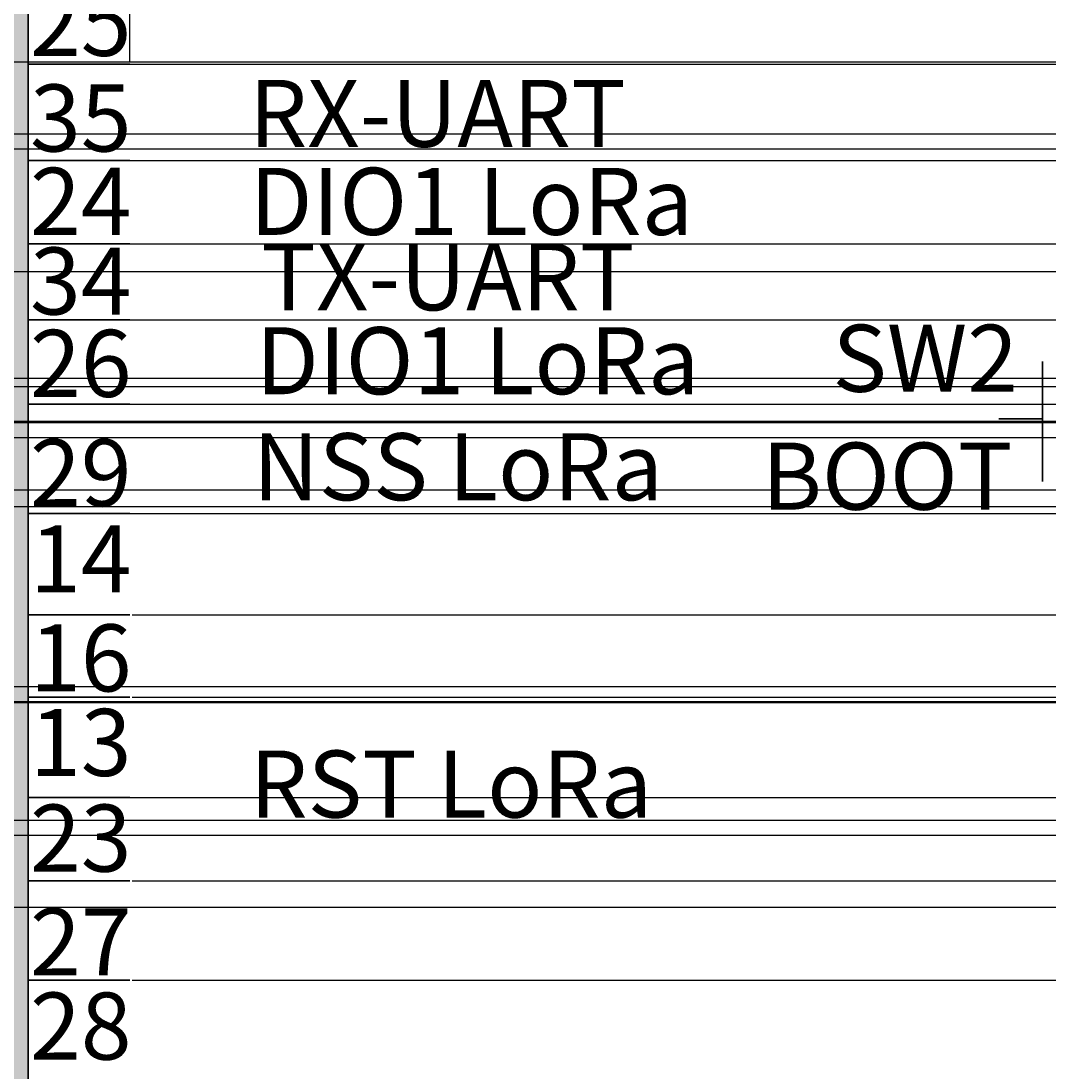
# Model space of a CAD drawing. Units: inches. Extents: x 23 to 132, y 5 to 105.
# Tile 10 of 14: x 81 to 107, y 50 to 77. Entities that reach past the tile are written whole.
import ezdxf

# ---------------------------------------------------------------- set-up
doc = ezdxf.new("R2010")
doc.units = ezdxf.units.IN
doc.header["$MEASUREMENT"] = 0
for name, color, linetype, lineweight in [('A-ANNO-DIMS', 2, 'Continuous', 18), ('E-ANNO-IDEN', 4, 'Continuous', 18), ('E-ANNO-NETL', 30, 'Continuous', 18), ('E-ANNO-TEXT', 3, 'Continuous', 18), ('E-SYMB', 1, 'Continuous', 35), ('E-SYMB-PATT', 1, 'Continuous', 18), ('E-WIRE', 3, 'Continuous', 25)]:
    doc.layers.add(name, color=color, linetype=linetype, lineweight=lineweight)
doc.styles.get("Standard").update_dxf_attribs({"font": 'arial.ttf'})
doc.dimstyles.get("Standard").update_dxf_attribs({"dimtxt": 0.18, "dimasz": 0.18, "dimexe": 0.18, "dimexo": 0.0625, "dimgap": 0.09, "dimtad": 0, "dimtih": 1, "dimtoh": 1, "dimdec": 4, "dimzin": 0, "dimdsep": 46, "dimtxsty": 'Standard', "dimcen": 0.09, "dimadec": 0, "dimazin": 0, "dimtfac": 1, "dimtdec": 4, "dimtofl": 0, "dimtmove": 0, "dimatfit": 3, "dimfxl": 1, "dimtolj": 1, "dimtzin": 0, "dimarcsym": 0})

# ---------------------------------------------------------------- blocks, each defined once
blk = doc.blocks.new('*D2')
at = {"layer": 'A-ANNO-DIMS', "color": 0, "lineweight": -2, "transparency": 16777216}
for p, q in [((28.697, 66.272), (28.697, 105.232)), ((123.211, 99.539), (123.211, 105.232)), ((28.877, 105.052), (75.577, 105.052)), ((123.031, 105.052), (76.33, 105.052))]:
    blk.add_line(p, q, dxfattribs=at)
at = {"layer": 'A-ANNO-DIMS', "color": 0, "transparency": 16777216}
for points in [[(28.877, 105.082), (28.877, 105.022), (28.697, 105.052)], [(123.031, 105.082), (123.031, 105.022), (123.211, 105.052)]]:
    blk.add_solid(points, dxfattribs=at)
at = {"layer": 'Defpoints', "color": 0, "transparency": 16777216}
for p in [(123.211, 105.052), (123.211, 99.477), (28.697, 66.21)]:
    blk.add_point(p, dxfattribs=at)
at = {"layer": 'A-ANNO-DIMS', "color": 0, "transparency": 16777216, "insert": (75.954, 105.052), "char_height": 0.18, "attachment_point": 5}
blk.add_mtext('\\A1;94.51', dxfattribs=at)
blk = doc.blocks.new('*D3')
at = {"layer": 'A-ANNO-DIMS', "color": 0, "lineweight": -2, "transparency": 16777216}
for p, q in [((121.409, 99.285), (129.239, 99.285)), ((129.059, 99.105), (129.059, 55.423)), ((129.059, 11.378), (129.059, 55.06)), ((72.981, 11.198), (129.239, 11.198))]:
    blk.add_line(p, q, dxfattribs=at)
at = {"layer": 'A-ANNO-DIMS', "color": 0, "transparency": 16777216}
for points in [[(129.029, 99.105), (129.089, 99.105), (129.059, 99.285)], [(129.029, 11.378), (129.089, 11.378), (129.059, 11.198)]]:
    blk.add_solid(points, dxfattribs=at)
at = {"layer": 'Defpoints', "color": 0, "transparency": 16777216}
for p in [(121.346, 99.285), (129.059, 99.285), (72.919, 11.198)]:
    blk.add_point(p, dxfattribs=at)
at = {"layer": 'A-ANNO-DIMS', "color": 0, "transparency": 16777216, "insert": (129.059, 55.241), "char_height": 0.18, "attachment_point": 5}
blk.add_mtext('\\A1;88.09', dxfattribs=at)
blk = doc.blocks.new('*D15')
at = {"layer": 'A-ANNO-DIMS', "color": 0, "lineweight": -2, "transparency": 16777216}
for p, q in [((50.327, 77.095), (129.239, 77.095)), ((129.059, 76.915), (129.059, 76.538)), ((129.059, 75.801), (129.059, 76.177)), ((47.783, 75.621), (129.239, 75.621))]:
    blk.add_line(p, q, dxfattribs=at)
at = {"layer": 'A-ANNO-DIMS', "color": 0, "transparency": 16777216}
for points in [[(129.029, 76.915), (129.089, 76.915), (129.059, 77.095)], [(129.029, 75.801), (129.089, 75.801), (129.059, 75.621)]]:
    blk.add_solid(points, dxfattribs=at)
at = {"layer": 'Defpoints', "color": 0, "transparency": 16777216}
for p in [(50.265, 77.095), (47.72, 75.621), (129.059, 75.621)]:
    blk.add_point(p, dxfattribs=at)
at = {"layer": 'A-ANNO-DIMS', "color": 0, "transparency": 16777216, "insert": (129.059, 76.358), "char_height": 0.18, "attachment_point": 5}
blk.add_mtext('\\A1;1.47', dxfattribs=at)
blk = doc.blocks.new('*D16')
at = {"layer": 'A-ANNO-DIMS', "color": 0, "lineweight": -2, "transparency": 16777216}
for p, q in [((47.783, 75.621), (129.239, 75.621)), ((129.059, 75.441), (129.059, 73.177)), ((129.059, 70.55), (129.059, 72.814)), ((47.783, 70.37), (129.239, 70.37))]:
    blk.add_line(p, q, dxfattribs=at)
at = {"layer": 'A-ANNO-DIMS', "color": 0, "transparency": 16777216}
for points in [[(129.029, 75.441), (129.089, 75.441), (129.059, 75.621)], [(129.029, 70.55), (129.089, 70.55), (129.059, 70.37)]]:
    blk.add_solid(points, dxfattribs=at)
at = {"layer": 'Defpoints', "color": 0, "transparency": 16777216}
for p in [(47.72, 75.621), (47.72, 70.37), (129.059, 70.37)]:
    blk.add_point(p, dxfattribs=at)
at = {"layer": 'A-ANNO-DIMS', "color": 0, "transparency": 16777216, "insert": (129.059, 72.996), "char_height": 0.18, "attachment_point": 5}
blk.add_mtext('\\A1;5.25', dxfattribs=at)
blk = doc.blocks.new('*D17')
at = {"layer": 'A-ANNO-DIMS', "color": 0, "lineweight": -2, "transparency": 16777216}
for p, q in [((47.783, 70.37), (129.239, 70.37)), ((129.059, 70.19), (129.059, 68.678)), ((129.059, 66.801), (129.059, 68.314)), ((47.783, 66.621), (129.239, 66.621))]:
    blk.add_line(p, q, dxfattribs=at)
at = {"layer": 'A-ANNO-DIMS', "color": 0, "transparency": 16777216}
for points in [[(129.029, 70.19), (129.089, 70.19), (129.059, 70.37)], [(129.029, 66.801), (129.089, 66.801), (129.059, 66.621)]]:
    blk.add_solid(points, dxfattribs=at)
at = {"layer": 'Defpoints', "color": 0, "transparency": 16777216}
for p in [(47.72, 70.37), (47.72, 66.621), (129.059, 66.621)]:
    blk.add_point(p, dxfattribs=at)
at = {"layer": 'A-ANNO-DIMS', "color": 0, "transparency": 16777216, "insert": (129.059, 68.496), "char_height": 0.18, "attachment_point": 5}
blk.add_mtext('\\A1;3.75', dxfattribs=at)
blk = doc.blocks.new('*D24')
at = {"layer": 'A-ANNO-DIMS', "color": 0, "lineweight": -2, "transparency": 16777216}
for p, q in [((81.032, 77.095), (129.239, 77.095)), ((129.059, 76.915), (129.059, 76.509)), ((129.059, 75.739), (129.059, 76.145)), ((83.576, 75.559), (129.239, 75.559))]:
    blk.add_line(p, q, dxfattribs=at)
at = {"layer": 'A-ANNO-DIMS', "color": 0, "transparency": 16777216}
for points in [[(129.029, 76.915), (129.089, 76.915), (129.059, 77.095)], [(129.029, 75.739), (129.089, 75.739), (129.059, 75.559)]]:
    blk.add_solid(points, dxfattribs=at)
at = {"layer": 'Defpoints', "color": 0, "transparency": 16777216}
for p in [(80.969, 77.095), (83.514, 75.559), (129.059, 75.559)]:
    blk.add_point(p, dxfattribs=at)
at = {"layer": 'A-ANNO-DIMS', "color": 0, "transparency": 16777216, "insert": (129.059, 76.327), "char_height": 0.18, "attachment_point": 5}
blk.add_mtext('\\A1;1.54', dxfattribs=at)
blk = doc.blocks.new('*D25')
at = {"layer": 'A-ANNO-DIMS', "color": 0, "lineweight": -2, "transparency": 16777216}
for p, q in [((83.576, 75.559), (129.239, 75.559)), ((129.059, 75.379), (129.059, 74.534)), ((129.059, 73.327), (129.059, 74.173)), ((83.576, 73.147), (129.239, 73.147))]:
    blk.add_line(p, q, dxfattribs=at)
at = {"layer": 'A-ANNO-DIMS', "color": 0, "transparency": 16777216}
for points in [[(129.029, 75.379), (129.089, 75.379), (129.059, 75.559)], [(129.029, 73.327), (129.089, 73.327), (129.059, 73.147)]]:
    blk.add_solid(points, dxfattribs=at)
at = {"layer": 'Defpoints', "color": 0, "transparency": 16777216}
for p in [(83.514, 75.559), (83.514, 73.147), (129.059, 73.147)]:
    blk.add_point(p, dxfattribs=at)
at = {"layer": 'A-ANNO-DIMS', "color": 0, "transparency": 16777216, "insert": (129.059, 74.353), "char_height": 0.18, "attachment_point": 5}
blk.add_mtext('\\A1;2.41', dxfattribs=at)
blk = doc.blocks.new('*D26')
at = {"layer": 'A-ANNO-DIMS', "color": 0, "lineweight": -2, "transparency": 16777216}
for p, q in [((83.576, 73.147), (129.239, 73.147)), ((129.059, 72.967), (129.059, 72.286)), ((129.059, 71.241), (129.059, 71.922)), ((83.576, 71.061), (129.239, 71.061))]:
    blk.add_line(p, q, dxfattribs=at)
at = {"layer": 'A-ANNO-DIMS', "color": 0, "transparency": 16777216}
for points in [[(129.029, 72.967), (129.089, 72.967), (129.059, 73.147)], [(129.029, 71.241), (129.089, 71.241), (129.059, 71.061)]]:
    blk.add_solid(points, dxfattribs=at)
at = {"layer": 'Defpoints', "color": 0, "transparency": 16777216}
for p in [(83.514, 73.147), (83.514, 71.061), (129.059, 71.061)]:
    blk.add_point(p, dxfattribs=at)
at = {"layer": 'A-ANNO-DIMS', "color": 0, "transparency": 16777216, "insert": (129.059, 72.104), "char_height": 0.18, "attachment_point": 5}
blk.add_mtext('\\A1;2.09', dxfattribs=at)
blk = doc.blocks.new('*D27')
at = {"layer": 'A-ANNO-DIMS', "color": 0, "lineweight": -2, "transparency": 16777216}
for p, q in [((83.576, 71.061), (129.239, 71.061)), ((129.059, 70.881), (129.059, 70.292)), ((129.059, 69.338), (129.059, 69.928)), ((83.576, 69.158), (129.239, 69.158))]:
    blk.add_line(p, q, dxfattribs=at)
at = {"layer": 'A-ANNO-DIMS', "color": 0, "transparency": 16777216}
for points in [[(129.029, 70.881), (129.089, 70.881), (129.059, 71.061)], [(129.029, 69.338), (129.089, 69.338), (129.059, 69.158)]]:
    blk.add_solid(points, dxfattribs=at)
at = {"layer": 'Defpoints', "color": 0, "transparency": 16777216}
for p in [(83.514, 71.061), (83.514, 69.158), (129.059, 69.158)]:
    blk.add_point(p, dxfattribs=at)
at = {"layer": 'A-ANNO-DIMS', "color": 0, "transparency": 16777216, "insert": (129.059, 70.11), "char_height": 0.18, "attachment_point": 5}
blk.add_mtext('\\A1;1.90', dxfattribs=at)
blk = doc.blocks.new('*D28')
at = {"layer": 'A-ANNO-DIMS', "color": 0, "lineweight": -2, "transparency": 16777216}
for p, q in [((83.576, 69.158), (129.239, 69.158)), ((129.059, 68.978), (129.059, 68.282)), ((129.059, 67.226), (129.059, 67.922)), ((83.576, 67.046), (129.239, 67.046))]:
    blk.add_line(p, q, dxfattribs=at)
at = {"layer": 'A-ANNO-DIMS', "color": 0, "transparency": 16777216}
for points in [[(129.029, 68.978), (129.089, 68.978), (129.059, 69.158)], [(129.029, 67.226), (129.089, 67.226), (129.059, 67.046)]]:
    blk.add_solid(points, dxfattribs=at)
at = {"layer": 'Defpoints', "color": 0, "transparency": 16777216}
for p in [(83.514, 69.158), (83.514, 67.046), (129.059, 67.046)]:
    blk.add_point(p, dxfattribs=at)
at = {"layer": 'A-ANNO-DIMS', "color": 0, "transparency": 16777216, "insert": (129.059, 68.102), "char_height": 0.18, "attachment_point": 5}
blk.add_mtext('\\A1;2.112', dxfattribs=at)
blk = doc.blocks.new('*D29')
at = {"layer": 'A-ANNO-DIMS', "color": 0, "lineweight": -2, "transparency": 16777216}
for p, q in [((83.576, 67.046), (129.239, 67.046)), ((129.059, 66.866), (129.059, 65.855)), ((129.059, 64.482), (129.059, 65.494)), ((83.576, 64.302), (129.239, 64.302))]:
    blk.add_line(p, q, dxfattribs=at)
at = {"layer": 'A-ANNO-DIMS', "color": 0, "transparency": 16777216}
for points in [[(129.029, 66.866), (129.089, 66.866), (129.059, 67.046)], [(129.029, 64.482), (129.089, 64.482), (129.059, 64.302)]]:
    blk.add_solid(points, dxfattribs=at)
at = {"layer": 'Defpoints', "color": 0, "transparency": 16777216}
for p in [(83.514, 67.046), (83.514, 64.302), (129.059, 64.302)]:
    blk.add_point(p, dxfattribs=at)
at = {"layer": 'A-ANNO-DIMS', "color": 0, "transparency": 16777216, "insert": (129.059, 65.674), "char_height": 0.18, "attachment_point": 5}
blk.add_mtext('\\A1;2.744', dxfattribs=at)
blk = doc.blocks.new('*D30')
at = {"layer": 'A-ANNO-DIMS', "color": 0, "lineweight": -2, "transparency": 16777216}
for p, q in [((83.576, 64.302), (129.239, 64.302)), ((129.059, 64.122), (129.059, 63.217)), ((129.059, 61.949), (129.059, 62.853)), ((83.576, 61.769), (129.239, 61.769))]:
    blk.add_line(p, q, dxfattribs=at)
at = {"layer": 'A-ANNO-DIMS', "color": 0, "transparency": 16777216}
for points in [[(129.029, 64.122), (129.089, 64.122), (129.059, 64.302)], [(129.029, 61.949), (129.089, 61.949), (129.059, 61.769)]]:
    blk.add_solid(points, dxfattribs=at)
at = {"layer": 'Defpoints', "color": 0, "transparency": 16777216}
for p in [(83.514, 64.302), (83.514, 61.769), (129.059, 61.769)]:
    blk.add_point(p, dxfattribs=at)
at = {"layer": 'A-ANNO-DIMS', "color": 0, "transparency": 16777216, "insert": (129.059, 63.035), "char_height": 0.18, "attachment_point": 5}
blk.add_mtext('\\A1;2.53', dxfattribs=at)
blk = doc.blocks.new('*D31')
at = {"layer": 'A-ANNO-DIMS', "color": 0, "lineweight": -2, "transparency": 16777216}
for p, q in [((83.576, 61.769), (129.239, 61.769)), ((129.059, 61.589), (129.059, 60.918)), ((129.059, 59.883), (129.059, 60.554)), ((83.576, 59.703), (129.239, 59.703))]:
    blk.add_line(p, q, dxfattribs=at)
at = {"layer": 'A-ANNO-DIMS', "color": 0, "transparency": 16777216}
for points in [[(129.029, 61.589), (129.089, 61.589), (129.059, 61.769)], [(129.029, 59.883), (129.089, 59.883), (129.059, 59.703)]]:
    blk.add_solid(points, dxfattribs=at)
at = {"layer": 'Defpoints', "color": 0, "transparency": 16777216}
for p in [(83.514, 61.769), (83.514, 59.703), (129.059, 59.703)]:
    blk.add_point(p, dxfattribs=at)
at = {"layer": 'A-ANNO-DIMS', "color": 0, "transparency": 16777216, "insert": (129.059, 60.736), "char_height": 0.18, "attachment_point": 5}
blk.add_mtext('\\A1;2.07', dxfattribs=at)
blk = doc.blocks.new('*D32')
at = {"layer": 'A-ANNO-DIMS', "color": 0, "lineweight": -2, "transparency": 16777216}
for p, q in [((83.576, 59.703), (129.239, 59.703)), ((129.059, 59.523), (129.059, 58.629)), ((129.059, 57.372), (129.059, 58.266)), ((83.576, 57.192), (129.239, 57.192))]:
    blk.add_line(p, q, dxfattribs=at)
at = {"layer": 'A-ANNO-DIMS', "color": 0, "transparency": 16777216}
for points in [[(129.029, 59.523), (129.089, 59.523), (129.059, 59.703)], [(129.029, 57.372), (129.089, 57.372), (129.059, 57.192)]]:
    blk.add_solid(points, dxfattribs=at)
at = {"layer": 'Defpoints', "color": 0, "transparency": 16777216}
for p in [(83.514, 59.703), (83.514, 57.192), (129.059, 57.192)]:
    blk.add_point(p, dxfattribs=at)
at = {"layer": 'A-ANNO-DIMS', "color": 0, "transparency": 16777216, "insert": (129.059, 58.447), "char_height": 0.18, "attachment_point": 5}
blk.add_mtext('\\A1;2.51', dxfattribs=at)
blk = doc.blocks.new('*D33')
at = {"layer": 'A-ANNO-DIMS', "color": 0, "lineweight": -2, "transparency": 16777216}
for p, q in [((83.576, 57.192), (129.239, 57.192)), ((129.059, 57.012), (129.059, 56.33)), ((129.059, 55.284), (129.059, 55.966)), ((83.576, 55.104), (129.239, 55.104))]:
    blk.add_line(p, q, dxfattribs=at)
at = {"layer": 'A-ANNO-DIMS', "color": 0, "transparency": 16777216}
for points in [[(129.029, 57.012), (129.089, 57.012), (129.059, 57.192)], [(129.029, 55.284), (129.089, 55.284), (129.059, 55.104)]]:
    blk.add_solid(points, dxfattribs=at)
at = {"layer": 'Defpoints', "color": 0, "transparency": 16777216}
for p in [(83.514, 57.192), (83.514, 55.104), (129.059, 55.104)]:
    blk.add_point(p, dxfattribs=at)
at = {"layer": 'A-ANNO-DIMS', "color": 0, "transparency": 16777216, "insert": (129.059, 56.148), "char_height": 0.18, "attachment_point": 5}
blk.add_mtext('\\A1;2.09', dxfattribs=at)
blk = doc.blocks.new('*D34')
at = {"layer": 'A-ANNO-DIMS', "color": 0, "lineweight": -2, "transparency": 16777216}
for p, q in [((83.576, 55.104), (129.239, 55.104)), ((129.059, 54.924), (129.059, 54.042)), ((129.059, 52.797), (129.059, 53.678)), ((83.576, 52.617), (129.239, 52.617))]:
    blk.add_line(p, q, dxfattribs=at)
at = {"layer": 'A-ANNO-DIMS', "color": 0, "transparency": 16777216}
for points in [[(129.029, 54.924), (129.089, 54.924), (129.059, 55.104)], [(129.029, 52.797), (129.089, 52.797), (129.059, 52.617)]]:
    blk.add_solid(points, dxfattribs=at)
at = {"layer": 'Defpoints', "color": 0, "transparency": 16777216}
for p in [(83.514, 55.104), (83.514, 52.617), (129.059, 52.617)]:
    blk.add_point(p, dxfattribs=at)
at = {"layer": 'A-ANNO-DIMS', "color": 0, "transparency": 16777216, "insert": (129.059, 53.86), "char_height": 0.18, "attachment_point": 5}
blk.add_mtext('\\A1;2.49', dxfattribs=at)
blk = doc.blocks.new('*D35')
at = {"layer": 'A-ANNO-DIMS', "color": 0, "lineweight": -2, "transparency": 16777216}
for p, q in [((83.576, 52.617), (129.239, 52.617)), ((129.059, 52.437), (129.059, 51.532)), ((129.059, 50.264), (129.059, 51.168)), ((83.576, 50.084), (129.239, 50.084))]:
    blk.add_line(p, q, dxfattribs=at)
at = {"layer": 'A-ANNO-DIMS', "color": 0, "transparency": 16777216}
for points in [[(129.029, 52.437), (129.089, 52.437), (129.059, 52.617)], [(129.029, 50.264), (129.089, 50.264), (129.059, 50.084)]]:
    blk.add_solid(points, dxfattribs=at)
at = {"layer": 'Defpoints', "color": 0, "transparency": 16777216}
for p in [(83.514, 52.617), (83.514, 50.084), (129.059, 50.084)]:
    blk.add_point(p, dxfattribs=at)
at = {"layer": 'A-ANNO-DIMS', "color": 0, "transparency": 16777216, "insert": (129.059, 51.35), "char_height": 0.18, "attachment_point": 5}
blk.add_mtext('\\A1;2.53', dxfattribs=at)
blk = doc.blocks.new('*D49')
at = {"layer": 'A-ANNO-DIMS', "color": 0, "lineweight": -2, "transparency": 16777216}
for p, q in [((83.514, 75.622), (83.514, 105.232)), ((107.287, 75.622), (107.287, 105.232)), ((83.694, 105.052), (94.936, 105.052)), ((107.107, 105.052), (95.865, 105.052))]:
    blk.add_line(p, q, dxfattribs=at)
at = {"layer": 'A-ANNO-DIMS', "color": 0, "transparency": 16777216}
for points in [[(83.694, 105.082), (83.694, 105.022), (83.514, 105.052)], [(107.107, 105.082), (107.107, 105.022), (107.287, 105.052)]]:
    blk.add_solid(points, dxfattribs=at)
at = {"layer": 'Defpoints', "color": 0, "transparency": 16777216}
for p in [(107.287, 105.052), (83.514, 75.559), (107.287, 75.559)]:
    blk.add_point(p, dxfattribs=at)
at = {"layer": 'A-ANNO-DIMS', "color": 0, "transparency": 16777216, "insert": (95.4, 105.052), "char_height": 0.18, "attachment_point": 5}
blk.add_mtext('\\A1;23.774', dxfattribs=at)
blk = doc.blocks.new('*D57')
at = {"layer": 'A-ANNO-DIMS', "color": 0, "lineweight": -2, "transparency": 16777216}
for p, q in [((30.358, 64.901), (129.239, 64.901)), ((129.059, 64.721), (129.059, 62.62)), ((129.059, 60.155), (129.059, 62.256)), ((30.358, 59.975), (129.239, 59.975))]:
    blk.add_line(p, q, dxfattribs=at)
at = {"layer": 'A-ANNO-DIMS', "color": 0, "transparency": 16777216}
for points in [[(129.029, 64.721), (129.089, 64.721), (129.059, 64.901)], [(129.029, 60.155), (129.089, 60.155), (129.059, 59.975)]]:
    blk.add_solid(points, dxfattribs=at)
at = {"layer": 'Defpoints', "color": 0, "transparency": 16777216}
for p in [(30.295, 64.901), (129.059, 64.901), (30.295, 59.975)]:
    blk.add_point(p, dxfattribs=at)
at = {"layer": 'A-ANNO-DIMS', "color": 0, "transparency": 16777216, "insert": (129.059, 62.438), "char_height": 0.18, "attachment_point": 5}
blk.add_mtext('\\A1;4.925', dxfattribs=at)
blk = doc.blocks.new('*D58')
at = {"layer": 'A-ANNO-DIMS', "color": 0, "lineweight": -2, "transparency": 16777216}
for p, q in [((30.358, 73.814), (129.239, 73.814)), ((129.059, 73.634), (129.059, 70.194)), ((129.059, 66.39), (129.059, 69.83)), ((30.359, 66.21), (129.239, 66.21))]:
    blk.add_line(p, q, dxfattribs=at)
at = {"layer": 'A-ANNO-DIMS', "color": 0, "transparency": 16777216}
for points in [[(129.029, 73.634), (129.089, 73.634), (129.059, 73.814)], [(129.029, 66.39), (129.089, 66.39), (129.059, 66.21)]]:
    blk.add_solid(points, dxfattribs=at)
at = {"layer": 'Defpoints', "color": 0, "transparency": 16777216}
for p in [(30.295, 73.814), (129.059, 73.814), (30.297, 66.21)]:
    blk.add_point(p, dxfattribs=at)
at = {"layer": 'A-ANNO-DIMS', "color": 0, "transparency": 16777216, "insert": (129.059, 70.012), "char_height": 0.18, "attachment_point": 5}
blk.add_mtext('\\A1;7.604', dxfattribs=at)
blk = doc.blocks.new('*D65')
at = {"layer": 'A-ANNO-DIMS', "color": 0, "lineweight": -2, "transparency": 16777216}
for p, q in [((38.414, 67.485), (129.239, 67.485)), ((129.059, 67.305), (129.059, 66.165)), ((129.059, 64.66), (129.059, 65.801)), ((38.414, 64.48), (129.239, 64.48))]:
    blk.add_line(p, q, dxfattribs=at)
at = {"layer": 'A-ANNO-DIMS', "color": 0, "transparency": 16777216}
for points in [[(129.029, 67.305), (129.089, 67.305), (129.059, 67.485)], [(129.029, 64.66), (129.089, 64.66), (129.059, 64.48)]]:
    blk.add_solid(points, dxfattribs=at)
at = {"layer": 'Defpoints', "color": 0, "transparency": 16777216}
for p in [(38.351, 67.485), (129.059, 67.485), (38.351, 64.48)]:
    blk.add_point(p, dxfattribs=at)
at = {"layer": 'A-ANNO-DIMS', "color": 0, "transparency": 16777216, "insert": (129.059, 65.983), "char_height": 0.18, "attachment_point": 5}
blk.add_mtext('\\A1;3.005', dxfattribs=at)
blk = doc.blocks.new('*D70')
at = {"layer": 'A-ANNO-DIMS', "color": 0, "lineweight": -2, "transparency": 16777216}
for p, q in [((35.392, 56.625), (129.239, 56.625)), ((129.059, 56.445), (129.059, 55.716)), ((129.059, 54.624), (129.059, 55.352)), ((33.892, 54.444), (129.239, 54.444))]:
    blk.add_line(p, q, dxfattribs=at)
at = {"layer": 'A-ANNO-DIMS', "color": 0, "transparency": 16777216}
for points in [[(129.029, 56.445), (129.089, 56.445), (129.059, 56.625)], [(129.029, 54.624), (129.089, 54.624), (129.059, 54.444)]]:
    blk.add_solid(points, dxfattribs=at)
at = {"layer": 'Defpoints', "color": 0, "transparency": 16777216}
for p in [(35.33, 56.625), (33.83, 54.444), (129.059, 54.444)]:
    blk.add_point(p, dxfattribs=at)
at = {"layer": 'A-ANNO-DIMS', "color": 0, "transparency": 16777216, "insert": (129.059, 55.534), "char_height": 0.18, "attachment_point": 5}
blk.add_mtext('\\A1;2.18', dxfattribs=at)
blk = doc.blocks.new('*D78')
at = {"layer": 'A-ANNO-DIMS', "color": 0, "lineweight": -2, "transparency": 16777216}
for p, q in [((112.773, 67.688), (22.942, 67.688)), ((23.122, 67.508), (23.122, 67.314)), ((23.122, 66.759), (23.122, 66.953)), ((112.773, 66.579), (22.942, 66.579))]:
    blk.add_line(p, q, dxfattribs=at)
at = {"layer": 'A-ANNO-DIMS', "color": 0, "transparency": 16777216}
for points in [[(23.092, 67.508), (23.152, 67.508), (23.122, 67.688)], [(23.092, 66.759), (23.152, 66.759), (23.122, 66.579)]]:
    blk.add_solid(points, dxfattribs=at)
at = {"layer": 'Defpoints', "color": 0, "transparency": 16777216}
for p in [(23.122, 67.688), (112.835, 67.688), (112.835, 66.579)]:
    blk.add_point(p, dxfattribs=at)
at = {"layer": 'A-ANNO-DIMS', "color": 0, "transparency": 16777216, "insert": (23.122, 67.133), "char_height": 0.18, "attachment_point": 5}
blk.add_mtext('\\A1;1.11', dxfattribs=at)
blk = doc.blocks.new('*D79')
at = {"layer": 'A-ANNO-DIMS', "color": 0, "lineweight": -2, "transparency": 16777216}
for p, q in [((114.373, 66.579), (22.942, 66.579)), ((23.122, 66.399), (23.122, 63.267)), ((23.122, 59.77), (23.122, 62.903)), ((114.371, 59.59), (22.942, 59.59))]:
    blk.add_line(p, q, dxfattribs=at)
at = {"layer": 'A-ANNO-DIMS', "color": 0, "transparency": 16777216}
for points in [[(23.092, 66.399), (23.152, 66.399), (23.122, 66.579)], [(23.092, 59.77), (23.152, 59.77), (23.122, 59.59)]]:
    blk.add_solid(points, dxfattribs=at)
at = {"layer": 'Defpoints', "color": 0, "transparency": 16777216}
for p in [(23.122, 66.579), (114.435, 66.579), (114.434, 59.59)]:
    blk.add_point(p, dxfattribs=at)
at = {"layer": 'A-ANNO-DIMS', "color": 0, "transparency": 16777216, "insert": (23.122, 63.085), "char_height": 0.18, "attachment_point": 5}
blk.add_mtext('\\A1;6.988', dxfattribs=at)
blk = doc.blocks.new('*D80')
at = {"layer": 'A-ANNO-DIMS', "color": 0, "lineweight": -2, "transparency": 16777216}
for p, q in [((114.373, 73.429), (22.942, 73.429)), ((23.122, 73.249), (23.122, 70.741)), ((23.122, 67.868), (23.122, 70.377)), ((114.373, 67.688), (22.942, 67.688))]:
    blk.add_line(p, q, dxfattribs=at)
at = {"layer": 'A-ANNO-DIMS', "color": 0, "transparency": 16777216}
for points in [[(23.092, 73.249), (23.152, 73.249), (23.122, 73.429)], [(23.092, 67.868), (23.152, 67.868), (23.122, 67.688)]]:
    blk.add_solid(points, dxfattribs=at)
at = {"layer": 'Defpoints', "color": 0, "transparency": 16777216}
for p in [(23.122, 73.429), (114.435, 73.429), (114.435, 67.688)]:
    blk.add_point(p, dxfattribs=at)
at = {"layer": 'A-ANNO-DIMS', "color": 0, "transparency": 16777216, "insert": (23.122, 70.559), "char_height": 0.18, "attachment_point": 5}
blk.add_mtext('\\A1;5.741', dxfattribs=at)
blk = doc.blocks.new('*D81')
at = {"layer": 'A-ANNO-DIMS', "color": 0, "lineweight": -2, "transparency": 16777216}
for p, q in [((110.705, 59.566), (22.942, 59.566)), ((23.122, 59.386), (23.122, 58.085)), ((23.122, 56.42), (23.122, 57.721)), ((110.759, 56.24), (22.942, 56.24))]:
    blk.add_line(p, q, dxfattribs=at)
at = {"layer": 'A-ANNO-DIMS', "color": 0, "transparency": 16777216}
for points in [[(23.092, 59.386), (23.152, 59.386), (23.122, 59.566)], [(23.092, 56.42), (23.152, 56.42), (23.122, 56.24)]]:
    blk.add_solid(points, dxfattribs=at)
at = {"layer": 'Defpoints', "color": 0, "transparency": 16777216}
for p in [(23.122, 59.566), (110.768, 59.566), (110.822, 56.24)]:
    blk.add_point(p, dxfattribs=at)
at = {"layer": 'A-ANNO-DIMS', "color": 0, "transparency": 16777216, "insert": (23.122, 57.903), "char_height": 0.18, "attachment_point": 5}
blk.add_mtext('\\A1;3.326', dxfattribs=at)

msp = doc.modelspace()

# ---------------------------------------------------------------- hatches: boundary and pattern name
at = {"layer": 'E-SYMB-PATT'}
h = msp.add_hatch(color=256, dxfattribs=at)
h.dxf.hatch_style = 1
h.paths.add_polyline_path([(80.9692, 77.095), (50.2646, 77.095), (50.2646, 18.0066), (80.9692, 18.0066)])

# ---------------------------------------------------------------- linework, layer by layer
at = {"layer": 'E-SYMB'}
for p, q in [((80.9692, 75.5594), (83.5136, 75.5594)), ((80.9692, 73.1469), (83.5136, 73.1469)), ((80.9692, 71.0614), (83.5136, 71.0614)), ((80.9692, 69.158), (83.5136, 69.158)), ((106.3748, 68.1087), (106.3748, 65.1036)), ((80.9692, 67.0462), (83.5136, 67.0462)), ((106.3748, 66.6754), (105.2796, 66.6754)), ((80.9692, 64.3021), (83.5136, 64.3021)), ((80.9692, 61.7685), (83.5136, 61.7685)), ((80.9692, 59.7032), (83.5136, 59.7032)), ((80.9692, 57.1918), (83.5136, 57.1918)), ((80.9692, 55.1036), (83.5136, 55.1036)), ((80.9692, 52.6172), (83.5136, 52.6172))]:
    msp.add_line(p, q, dxfattribs=at)
msp.add_lwpolyline([(50.2646, 77.095), (80.9692, 77.095), (80.9692, 18.0066), (50.2646, 18.0066)], close=True, dxfattribs=at)
at = {"layer": 'E-WIRE'}
for p, q in [((83.5136, 75.5594), (94.2651, 75.5594)), ((94.2651, 75.5594), (107.2874, 75.5594)), ((83.5136, 73.1469), (86.5493, 73.1469)), ((83.5136, 71.0614), (86.5493, 71.0614)), ((83.5136, 69.158), (86.5493, 69.158)), ((83.5136, 67.0462), (86.5493, 67.0462)), ((83.5136, 64.3021), (86.5493, 64.3021)), ((83.5136, 57.1918), (86.5493, 57.1918))]:
    msp.add_line(p, q, dxfattribs=at)

# ---------------------------------------------------------------- texts
at = {"layer": 'E-ANNO-IDEN'}
for s, p in [('SW2', (101.1109, 67.3537)), ('BOOT', (99.3463, 64.4007))]:
    msp.add_text(s, height=1.67943, dxfattribs=at).set_placement(p)
at = {"layer": 'E-ANNO-NETL'}
for s, p in [('RX-UART', (86.503, 73.488)), ('DIO1 LoRa', (86.5135, 71.2839)), ('TX-UART', (86.8044, 69.3952)), ('DIO1 LoRa', (86.6718, 67.2916)), ('NSS LoRa', (86.5913, 64.636)), ('RST LoRa', (86.5135, 56.6868))]:
    msp.add_text(s, height=1.67943, dxfattribs=at).set_placement(p)
at = {"layer": 'E-ANNO-TEXT'}
for s, p in [('25', (81.0136, 75.7678)), ('35', (81.0136, 73.3728)), ('24', (81.0136, 71.2848)), ('34', (81.0136, 69.2884)), ('26', (81.0136, 67.2244)), ('29', (81.0136, 64.4846)), ('14', (81.0136, 62.3268)), ('16', (81.0136, 59.8482)), ('13', (81.0136, 57.7301)), ('23', (81.0136, 55.3336)), ('27', (81.0136, 52.732)), ('28', (81.0136, 50.6249))]:
    msp.add_text(s, height=1.67943, dxfattribs=at).set_placement(p)

# ---------------------------------------------------------------- dimensions: what is measured, and where the dimension line sits
at = {"layer": 'A-ANNO-DIMS'}
for base, p1, p2, override, picture, middle in [((123.2107, 105.052), (28.6965, 66.2099), (123.2107, 99.477), {"dimdec": 2, "dimlfac": 1, "dimrnd": 0, "dimzin": 0, "dimdsep": 46, "dimlunit": 2}, '*D2', (75.9536, 105.052)), ((107.2874, 105.052), (83.5136, 75.5594), (107.2874, 75.5594), {"dimdec": 3, "dimlfac": 1, "dimrnd": 0, "dimzin": 0, "dimdsep": 46, "dimlunit": 2}, '*D49', (95.4005, 105.052))]:
    dim = msp.add_linear_dim(base=base, p1=p1, p2=p2, dimstyle='Standard', override=override, dxfattribs=at)
    dim.commit()
    dim.dimension.update_dxf_attribs({"geometry": picture, "text_midpoint": middle})
for base, p1, p2, override, picture, middle in [((129.0589, 99.2846), (72.9188, 11.1983), (121.3461, 99.2846), {"dimdec": 2, "dimlfac": 1, "dimrnd": 0, "dimzin": 0, "dimdsep": 46, "dimlunit": 2}, '*D3', (129.0589, 55.2415)), ((129.0589, 75.6207), (50.2646, 77.095), (47.7202, 75.6207), {"dimdec": 2, "dimlfac": 1, "dimrnd": 0, "dimzin": 0, "dimdsep": 46, "dimlunit": 2}, '*D15', (129.0589, 76.3579)), ((129.0589, 75.5594), (80.9692, 77.095), (83.5136, 75.5594), {"dimdec": 2, "dimlfac": 1, "dimrnd": 0, "dimzin": 0, "dimdsep": 46, "dimlunit": 2}, '*D24', (129.0589, 76.3272)), ((129.0589, 70.3705), (47.7202, 75.6207), (47.7202, 70.3705), {"dimdec": 2, "dimlfac": 1, "dimrnd": 0, "dimzin": 0, "dimdsep": 46, "dimlunit": 2}, '*D16', (129.0589, 72.9956)), ((129.0589, 73.1469), (83.5136, 75.5594), (83.5136, 73.1469), {"dimdec": 2, "dimlfac": 1, "dimrnd": 0, "dimzin": 0, "dimdsep": 46, "dimlunit": 2}, '*D25', (129.0589, 74.3532)), ((129.05891, 73.81438), (30.29652, 66.20989), (30.29537, 73.81438), {"dimdec": 3, "dimlfac": 1, "dimrnd": 0, "dimzin": 0, "dimdsep": 46, "dimlunit": 2}, '*D58', (129.05891, 70.01213)), ((23.1215, 73.4293), (114.4351, 67.6881), (114.4351, 73.4293), {"dimdec": 3, "dimlfac": 1, "dimrnd": 0, "dimzin": 0, "dimdsep": 46, "dimlunit": 2}, '*D80', (23.1215, 70.5587)), ((129.0589, 71.0614), (83.5136, 73.1469), (83.5136, 71.0614), {"dimdec": 2, "dimlfac": 1, "dimrnd": 0, "dimzin": 0, "dimdsep": 46, "dimlunit": 2}, '*D26', (129.0589, 72.1042)), ((129.0589, 69.158), (83.5136, 71.0614), (83.5136, 69.158), {"dimdec": 2, "dimlfac": 1, "dimrnd": 0, "dimzin": 0, "dimdsep": 46, "dimlunit": 2}, '*D27', (129.0589, 70.1097)), ((129.0589, 66.621), (47.7202, 70.3705), (47.7202, 66.621), {"dimdec": 2, "dimlfac": 1, "dimrnd": 0, "dimzin": 0, "dimdsep": 46, "dimlunit": 2}, '*D17', (129.0589, 68.4957)), ((129.0589, 67.0462), (83.5136, 69.158), (83.5136, 67.0462), {"dimdec": 3, "dimlfac": 1, "dimrnd": 0, "dimzin": 0, "dimdsep": 46, "dimlunit": 2}, '*D28', (129.0589, 68.1021)), ((23.1215, 67.6881), (112.8351, 66.5788), (112.8351, 67.6881), {"dimdec": 2, "dimlfac": 1, "dimrnd": 0, "dimzin": 0, "dimdsep": 46, "dimlunit": 2}, '*D78', (23.1215, 67.1334)), ((129.0589, 67.4851), (38.3512, 64.4801), (38.3512, 67.4851), {"dimdec": 3, "dimlfac": 1, "dimrnd": 0, "dimzin": 0, "dimdsep": 46, "dimlunit": 2}, '*D65', (129.0589, 65.9826)), ((129.0589, 64.3021), (83.5136, 67.0462), (83.5136, 64.3021), {"dimdec": 3, "dimlfac": 1, "dimrnd": 0, "dimzin": 0, "dimdsep": 46, "dimlunit": 2}, '*D29', (129.0589, 65.6741)), ((23.1215, 66.5788), (114.434, 59.5904), (114.4351, 66.5788), {"dimdec": 3, "dimlfac": 1, "dimrnd": 0, "dimzin": 0, "dimdsep": 46, "dimlunit": 2}, '*D79', (23.1215, 63.0846)), ((129.0589, 64.9007), (30.2954, 59.9755), (30.2954, 64.9007), {"dimdec": 3, "dimlfac": 1, "dimrnd": 0, "dimzin": 0, "dimdsep": 46, "dimlunit": 2}, '*D57', (129.0589, 62.4381)), ((129.0589, 61.7685), (83.5136, 64.3021), (83.5136, 61.7685), {"dimdec": 2, "dimlfac": 1, "dimrnd": 0, "dimzin": 0, "dimdsep": 46, "dimlunit": 2}, '*D30', (129.0589, 63.0353)), ((129.0589, 59.7032), (83.5136, 61.7685), (83.5136, 59.7032), {"dimdec": 2, "dimlfac": 1, "dimrnd": 0, "dimzin": 0, "dimdsep": 46, "dimlunit": 2}, '*D31', (129.0589, 60.7358)), ((23.1215, 59.566), (110.8219, 56.2399), (110.7677, 59.566), {"dimdec": 3, "dimlfac": 1, "dimrnd": 0, "dimzin": 0, "dimdsep": 46, "dimlunit": 2}, '*D81', (23.1215, 57.9029)), ((129.0589, 57.1918), (83.5136, 59.7032), (83.5136, 57.1918), {"dimdec": 2, "dimlfac": 1, "dimrnd": 0, "dimzin": 0, "dimdsep": 46, "dimlunit": 2}, '*D32', (129.0589, 58.4475)), ((129.0589, 55.1036), (83.5136, 57.1918), (83.5136, 55.1036), {"dimdec": 2, "dimlfac": 1, "dimrnd": 0, "dimzin": 0, "dimdsep": 46, "dimlunit": 2}, '*D33', (129.0589, 56.1477)), ((129.0589, 54.4437), (35.3299, 56.6249), (33.8299, 54.4437), {"dimdec": 2, "dimlfac": 1, "dimrnd": 0, "dimzin": 0, "dimdsep": 46, "dimlunit": 2}, '*D70', (129.0589, 55.5343)), ((129.0589, 52.6172), (83.5136, 55.1036), (83.5136, 52.6172), {"dimdec": 2, "dimlfac": 1, "dimrnd": 0, "dimzin": 0, "dimdsep": 46, "dimlunit": 2}, '*D34', (129.0589, 53.8604)), ((129.0589, 50.0837), (83.5136, 52.6172), (83.5136, 50.0837), {"dimdec": 2, "dimlfac": 1, "dimrnd": 0, "dimzin": 0, "dimdsep": 46, "dimlunit": 2}, '*D35', (129.0589, 51.3504))]:
    dim = msp.add_linear_dim(base=base, p1=p1, p2=p2, angle=90, dimstyle='Standard', override=override, dxfattribs=at)
    dim.commit()
    dim.dimension.update_dxf_attribs({"geometry": picture, "text_midpoint": middle})

doc.saveas('drawing.dxf')
